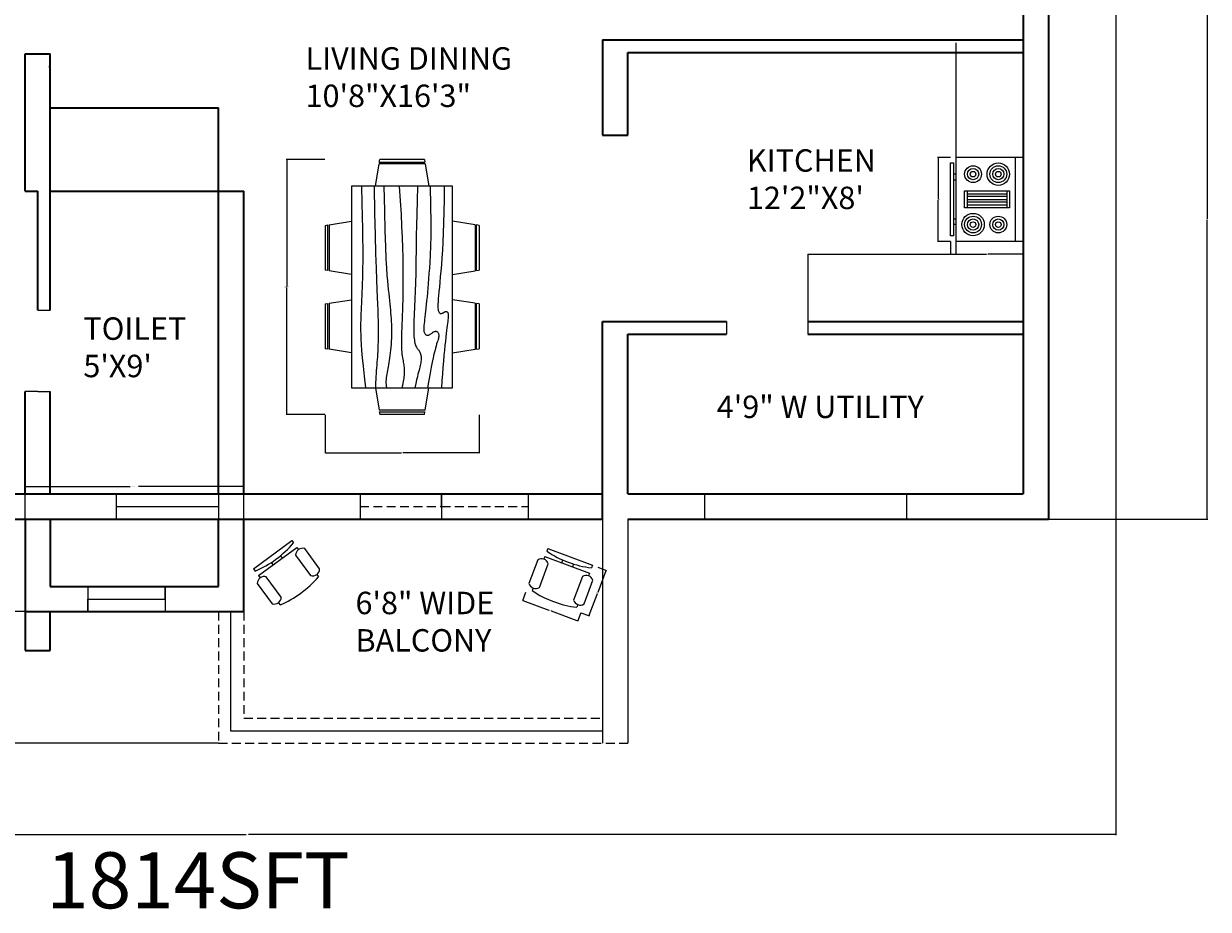
# Model space of a CAD drawing. Units: inches. Extents: x 514 to 1200, y -110 to 470.
# Tile 2 of 3: x 777 to 1200, y -110 to 206. Entities that reach past the tile are written whole.
import ezdxf

# ---------------------------------------------------------------- set-up
doc = ezdxf.new("R2010")
doc.units = ezdxf.units.IN
doc.linetypes.add('HIDDEN2', pattern=[4.7625, 3.175, -1.5875])
for name, color, linetype, lineweight in [('A-ANNO-DIMS', 2, 'Continuous', 18), ('A-ANNO-TEXT', 7, 'Continuous', 25), ('A-AREA-IDEN', 7, 'Continuous', 18), ('A-DOOR', 3, 'Continuous', 25), ('A-EQPM', 9, 'Continuous', 18), ('A-FLOR-FIXT', 9, 'Continuous', 18), ('A-FLOR-HIDN', 8, 'HIDDEN2', 18), ('A-FLOR-RAIL', 7, 'Continuous', 25), ('A-FURN', 8, 'Continuous', 18), ('A-GLAZ', 4, 'Continuous', 18), ('A-GLAZ-HIDN', 4, 'HIDDEN2', 18), ('A-WALL', 7, 'Continuous', 35)]:
    doc.layers.add(name, color=color, linetype=linetype, lineweight=lineweight)
doc.dimstyles.get("Standard").update_dxf_attribs({"dimtxt": 0.18, "dimasz": 0.18, "dimexe": 0.18, "dimexo": 0.0625, "dimgap": 0.09, "dimtad": 0, "dimtih": 1, "dimtoh": 1, "dimdec": 4, "dimzin": 0, "dimdsep": 46, "dimtxsty": 'Standard', "dimcen": 0.09, "dimadec": 0, "dimazin": 0, "dimtfac": 1, "dimtdec": 4, "dimtofl": 0, "dimtmove": 0, "dimatfit": 3, "dimfxl": 1, "dimtolj": 1, "dimtzin": 0, "dimarcsym": 0})

# ---------------------------------------------------------------- blocks, each defined once
blk = doc.blocks.new('Chair - Desk')
for p, q in [((-8.5, 0), (-8.5, -1)), ((-8.5, 0), (8.5, 0)), ((8.5, 0), (8.5, -1)), ((-8.5, -3), (-8.5, -4)), ((-8.5, -3), (8.5, -3)), ((-2, -3), (-2, -1.9355)), ((2, -1.9576), (2, -3)), ((8.5, -3), (8.5, -4)), ((-10.5, -5), (-10.5, -14)), ((-6.5, -14), (-6.5, -5)), ((6.5, -5), (6.5, -14)), ((10.5, -14), (10.5, -5)), ((-8.5, -15), (-8.5, -16)), ((8.5, -15), (8.5, -16))]:
    blk.add_line(p, q)
for centre, radius, start, end in [((-8.5, -6.5), 2.5, 36.8699, 143.1301), ((0, 34.625), 36.625, 256.5803, 283.4197), ((8.5, -6.5), 2.5, 36.8699, 143.1301), ((-8.5, -12.5), 2.5, 216.8699, 323.1301), ((0, 19.625), 36.625, 256.5803, 283.4197), ((8.5, -12.5), 2.5, 216.8699, 323.1301)]:
    blk.add_arc(centre, radius, start, end)
blk = doc.blocks.new('Dining Set - 36 x 72 in.')
for p, q in [((-22.2343, 26.00059), (-23.4847, 17.99762)), ((-22.2304, 26), (-5.7608, 26)), ((-22, 27.5), (-22.1562, 26.50042)), ((-5.8416, 26.5), (-22.1534, 26.5)), ((-22, 27.5), (-6, 27.5)), ((-5.8437, 26.49966), (-6, 27.5)), ((-4.5152, 17.99762), (-5.7655, 25.99926)), ((5.7657, 26.00059), (4.5153, 17.99762)), ((5.7696, 26), (22.2392, 26)), ((6, 27.5), (5.8438, 26.50042)), ((22.1584, 26.5), (5.8466, 26.5)), ((6, 27.5), (22, 27.5)), ((22.1563, 26.49966), (22, 27.5)), ((23.4848, 17.99762), (22.2345, 25.99926)), ((36, 18), (-36, 18)), ((-36, 18), (-36, -18)), ((36, -18), (36, 18)), ((-44.0006, 8.23428), (-35.9976, 9.48474)), ((44.0006, 8.23428), (35.9976, 9.48474)), ((-45.5, 8), (-44.5004, 8.15617)), ((-45.5, 8), (-45.5, -8)), ((-44.5, -8.15843), (-44.5, 8.15338)), ((-44, 8.23041), (-44, -8.23915)), ((44, 8.23041), (44, -8.23915)), ((44.5, -8.15843), (44.5, 8.15338)), ((45.5, 8), (44.5005, 8.15617)), ((45.5, 8), (45.5, -8)), ((-44.4997, -8.15631), (-45.5, -8)), ((-35.9976, -9.48476), (-43.9993, -8.2345)), ((35.9976, -9.48476), (43.9993, -8.2345)), ((44.4997, -8.15631), (45.5, -8)), ((-36, -18), (36, -18)), ((-22.2343, -26.0006), (-23.4847, -17.99762)), ((-4.5152, -17.99762), (-5.7655, -25.99928)), ((5.7657, -26.0006), (4.5153, -17.99762)), ((23.4848, -17.99762), (22.2345, -25.99928)), ((-22.2304, -26), (-5.7608, -26)), ((-22, -27.5), (-22.1562, -26.50044)), ((-5.8416, -26.5), (-22.1534, -26.5)), ((-22, -27.5), (-6, -27.5)), ((-5.8437, -26.49967), (-6, -27.5)), ((5.7696, -26), (22.2392, -26)), ((6, -27.5), (5.8438, -26.50044)), ((22.1584, -26.5), (5.8466, -26.5)), ((6, -27.5), (22, -27.5)), ((22.1563, -26.49967), (22, -27.5))]:
    blk.add_line(p, q)
for points in [[(-36, 15), (-31.1772, 14.97754), (-26.8079, 14.91406), (-22.8538, 14.81543), (-19.276, 14.6875), (-16.0362, 14.53613), (-13.0957, 14.36718), (-10.4159, 14.18652), (-7.9583, 14), (-5.6904, 13.81315), (-3.6035, 13.63021), (-1.6954, 13.45508), (0.0365, 13.29166), (1.5945, 13.14388), (2.9811, 13.01562), (4.1988, 12.9108), (5.25, 12.83333), (6.1393, 12.78613), (6.8802, 12.76823), (7.4883, 12.77767), (7.9792, 12.8125), (8.3685, 12.87077), (8.6719, 12.95052), (8.9049, 13.0498), (9.0833, 13.16666), (9.2205, 13.29899), (9.3216, 13.44401), (9.3895, 13.59879), (9.4271, 13.76041), (9.4373, 13.92594), (9.4232, 14.09245), (9.3875, 14.257), (9.3333, 14.41666), (9.2638, 14.56917), (9.1836, 14.71484), (9.0975, 14.85465), (9.0104, 14.98958), (8.9272, 15.1206), (8.8529, 15.2487), (8.7922, 15.37483), (8.75, 15.5), (8.7305, 15.62467), (8.7344, 15.74739), (8.7617, 15.86621), (8.8125, 15.97916), (8.8867, 16.08431), (8.9844, 16.17968), (9.1055, 16.26334), (9.25, 16.33333), (9.4189, 16.38802), (9.6172, 16.42708), (9.8506, 16.45052), (10.125, 16.45833), (10.4463, 16.45052), (10.8203, 16.42708), (11.2529, 16.38802), (11.75, 16.33333), (12.3184, 16.26318), (12.9694, 16.17838), (13.7151, 16.07991), (14.5677, 15.96875), (15.5395, 15.84586), (16.6426, 15.71224), (17.8893, 15.56884), (19.2917, 15.41666), (20.859, 15.25667), (22.5879, 15.08984), (24.4721, 14.91715), (26.5052, 14.73958), (28.6809, 14.5581), (30.9929, 14.3737), (33.4347, 14.18733), (36, 14)], [(-36, 10), (-28.9766, 10.14274), (-23.1725, 10.20442), (-18.4241, 10.19775), (-14.5677, 10.13541), (-11.4399, 10.03011), (-8.877, 9.89453), (-6.7154, 9.74137), (-4.7917, 9.58333), (-2.9698, 9.43082), (-1.2246, 9.28515), (0.4415, 9.14534), (2.026, 9.01041), (3.5266, 8.87939), (4.9408, 8.7513), (6.266, 8.62516), (7.5, 8.5), (8.6411, 8.37549), (9.6914, 8.2539), (10.6538, 8.13818), (11.5312, 8.03125), (12.3267, 7.93603), (13.043, 7.85547), (13.6831, 7.79248), (14.25, 7.75), (14.7471, 7.7303), (15.1797, 7.73307), (15.5537, 7.75732), (15.875, 7.80208), (16.1494, 7.86637), (16.3828, 7.94922), (16.5811, 8.04964), (16.75, 8.16666), (16.8944, 8.29915), (17.0143, 8.44531), (17.1089, 8.60319), (17.1771, 8.77083), (17.218, 8.94629), (17.2305, 9.1276), (17.2137, 9.31282), (17.1667, 9.5), (17.0895, 9.6875), (16.987, 9.875), (16.8649, 10.0625), (16.7292, 10.25), (16.5856, 10.4375), (16.4401, 10.625), (16.2985, 10.8125), (16.1667, 11), (16.05, 11.18733), (15.9518, 11.3737), (15.8752, 11.5581), (15.8229, 11.73958), (15.798, 11.91715), (15.8034, 12.08984), (15.842, 12.25667), (15.9167, 12.41666), (16.0295, 12.56836), (16.1784, 12.70833), (16.3605, 12.83268), (16.5729, 12.9375), (16.8127, 13.01888), (17.0768, 13.07291), (17.3625, 13.0957), (17.6667, 13.08333), (17.9894, 13.03312), (18.3418, 12.94726), (18.7382, 12.82918), (19.1927, 12.68229), (19.7195, 12.51001), (20.3327, 12.31575), (21.0465, 12.10294), (21.875, 11.875), (22.8357, 11.63354), (23.959, 11.37304), (25.2786, 11.08618), (26.8282, 10.76562), (28.6414, 10.40405), (30.752, 9.99414), (33.1936, 9.52856), (36, 9)], [(-36, 5.5), (-30.7157, 5.3348), (-26.069, 5.20963), (-21.9946, 5.11767), (-18.4271, 5.05208), (-15.3009, 5.00602), (-12.5508, 4.97265), (-10.1112, 4.94515), (-7.9167, 4.91666), (-5.909, 4.88167), (-4.0586, 4.83984), (-2.3429, 4.79215), (-0.7396, 4.73958), (0.7739, 4.6831), (2.22, 4.6237), (3.6213, 4.56233), (5, 4.5), (6.373, 4.43782), (7.7344, 4.3776), (9.0723, 4.32129), (10.375, 4.27083), (11.6309, 4.22819), (12.8281, 4.19531), (13.9551, 4.17415), (15, 4.16666), (15.954, 4.17448), (16.819, 4.19791), (17.6001, 4.23698), (18.3021, 4.29166), (18.9299, 4.36198), (19.4883, 4.44791), (19.9823, 4.54948), (20.4167, 4.66666), (20.7969, 4.79899), (21.1302, 4.94401), (21.4245, 5.09879), (21.6875, 5.26041), (21.9271, 5.42594), (22.1511, 5.59245), (22.3672, 5.757), (22.5834, 5.91666), (22.8065, 6.06868), (23.0404, 6.21093), (23.2879, 6.34147), (23.5521, 6.45833), (23.8358, 6.55957), (24.142, 6.64323), (24.4735, 6.70735), (24.8334, 6.75), (25.2235, 6.76969), (25.642, 6.76692), (26.0858, 6.74267), (26.5521, 6.69791), (27.0379, 6.63362), (27.5404, 6.55078), (28.0565, 6.45036), (28.5834, 6.33333), (29.1242, 6.19987), (29.7071, 6.04687), (30.3661, 5.87044), (31.1354, 5.66666), (32.0493, 5.43164), (33.142, 5.16146), (34.4475, 4.85221), (36, 4.5)], [(-36, -1), (-30.7915, -0.6591), (-26.0195, -0.38216), (-21.6519, -0.16284), (-17.6563, 0.00521), (-14.0005, 0.12833), (-10.6523, 0.21289), (-7.5796, 0.26522), (-4.75, 0.29166), (-2.134, 0.29793), (0.2878, 0.28711), (2.5317, 0.26163), (4.6146, 0.22396), (6.5529, 0.17651), (8.3633, 0.12174), (10.0623, 0.06209), (11.6667, 0), (13.1899, -0.06201), (14.6341, -0.1211), (15.9982, -0.17432), (17.2813, -0.21875), (18.4823, -0.25147), (19.6003, -0.26953), (20.6343, -0.27002), (21.5834, -0.25), (22.4481, -0.20768), (23.2357, -0.14584), (23.9549, -0.06836), (24.6146, 0.02083), (25.2235, 0.11784), (25.7904, 0.21875), (26.3241, 0.31966), (26.8334, 0.41666), (27.3265, 0.50618), (27.8099, 0.58593), (28.2894, 0.65397), (28.7709, 0.70833), (29.2601, 0.74707), (29.763, 0.76823), (30.2855, 0.76985), (30.8334, 0.75), (31.4088, 0.70784), (31.9994, 0.64713), (32.589, 0.57275), (33.1615, 0.48958), (33.7008, 0.4025), (34.1908, 0.3164), (34.6153, 0.23616), (34.9584, 0.16666), (35.2099, 0.11165), (35.3848, 0.07031), (35.504, 0.04069), (35.5886, 0.02083), (35.6594, 0.00879), (35.7377, 0.0026), (35.8442, 0.00032), (36, 0)], [(-36, -6.5), (-27.1843, -6.31267), (-20.084, -6.1263), (-14.469, -5.9419), (-10.1094, -5.76042), (-6.7752, -5.58285), (-4.2363, -5.41016), (-2.2629, -5.24333), (-0.625, -5.08334), (0.8708, -4.93099), (2.2715, -4.78646), (3.5872, -4.64974), (4.8281, -4.52084), (6.0046, -4.39974), (7.127, -4.28646), (8.2053, -4.18099), (9.25, -4.08334), (10.2705, -3.99382), (11.2734, -3.91407), (12.2647, -3.84603), (13.25, -3.79167), (14.2354, -3.75293), (15.2266, -3.73177), (16.2295, -3.73015), (17.25, -3.75), (18.2912, -3.79248), (19.3451, -3.85547), (20.4009, -3.93604), (21.4479, -4.03125), (22.4754, -4.13819), (23.4727, -4.25391), (24.4289, -4.37549), (25.3334, -4.5), (26.1785, -4.62492), (26.9694, -4.74935), (27.7145, -4.87281), (28.4219, -4.99479), (29.1, -5.11483), (29.7572, -5.23242), (30.4016, -5.34709), (31.0417, -5.45834), (31.6837, -5.56437), (32.3262, -5.65821), (32.9658, -5.73153), (33.599, -5.77604), (34.2224, -5.78345), (34.8327, -5.74545), (35.4264, -5.65373), (36, -5.5)], [(-36, -10), (-26.4022, -9.81299), (-18.4675, -9.62891), (-11.9839, -9.45069), (-6.7396, -9.28125), (-2.5226, -9.12354), (0.8789, -8.98047), (3.6769, -8.85498), (6.0833, -8.75), (8.2767, -8.66765), (10.3021, -8.60677), (12.1712, -8.56543), (13.8958, -8.54167), (15.4876, -8.53353), (16.9583, -8.53907), (18.3197, -8.55632), (19.5834, -8.58334), (20.7616, -8.61841), (21.8685, -8.66081), (22.9188, -8.71004), (23.9271, -8.76563), (24.9081, -8.82707), (25.8763, -8.89388), (26.8465, -8.96558), (27.8334, -9.04167), (28.8474, -9.12118), (29.8828, -9.20117), (30.93, -9.27824), (31.9792, -9.34896), (33.0205, -9.40991), (34.0443, -9.45768), (35.0407, -9.48885), (36, -9.5)], [(-36, -14.5), (-30.0881, -14.33513), (-25.0332, -14.21224), (-20.7312, -14.12647), (-17.0781, -14.07292), (-13.97, -14.04671), (-11.3027, -14.04297), (-8.9724, -14.05681), (-6.875, -14.08334), (-4.9224, -14.11833), (-3.0905, -14.16016), (-1.3709, -14.20785), (0.2448, -14.26042), (1.7647, -14.3169), (3.1973, -14.3763), (4.5507, -14.43767), (5.8333, -14.5), (7.0554, -14.5621), (8.235, -14.62175), (9.3922, -14.67652), (10.5469, -14.72396), (11.7192, -14.76164), (12.929, -14.78711), (14.1965, -14.79794), (15.5417, -14.79167), (16.9933, -14.76424), (18.6152, -14.70508), (20.4804, -14.60197), (22.6615, -14.44271), (25.2312, -14.21509), (28.2624, -13.9069), (31.8277, -13.50594), (36, -13)]]:
    blk.add_lwpolyline(points)
blk = doc.blocks.new('Range-Oven - 30 in top')
for p, q in [((0, -3), (30, -3)), ((12, -6), (18, -6)), ((13, -20), (13, -6)), ((14, -6), (14, -20)), ((15, -20), (15, -6)), ((16, -6), (16, -20)), ((17, -20), (17, -6)), ((18, -20), (12, -20)), ((6, -24), (6, -25)), ((8, -25), (8, -24)), ((22, -25), (22, -24)), ((24, -24), (24, -25))]:
    blk.add_line(p, q)
for points in [[(0, -24), (0, 0), (30, 0), (30, -24)], [(12, -21), (12, -5), (18, -5), (18, -21)], [(2, -26), (2, -25), (28, -25), (28, -26)]]:
    blk.add_lwpolyline(points, close=True)
for centre, radius in [((6, -9), 4), ((6, -9), 3), ((6, -9), 2), ((6, -9), 1), ((24, -9), 3), ((24, -9), 2), ((24, -9), 1), ((6, -18), 3), ((6, -18), 2), ((24, -18), 4), ((24, -18), 3), ((24, -18), 2), ((6, -18), 1), ((24, -18), 1)]:
    blk.add_circle(centre, radius)
blk = doc.blocks.new('WALL-BAY-60x24')
for p, q in [((0, 33), (0, 0)), ((9, 33), (9, 9)), ((69, 9), (69, 33)), ((78, 0), (78, 33)), ((9, 9), (69, 9)), ((0, 0), (78, 0))]:
    blk.add_line(p, q)
blk = doc.blocks.new('*D10')
at = {"layer": 'A-ANNO-DIMS', "color": 0, "lineweight": -2, "transparency": 16777216}
for p, q in [((956.39, 2.9), (955.25, -0.16)), ((955.48, -0.06), (964.67, -3.48)), ((974.82, -7.26), (965.64, -3.84)), ((976.07, -4.43), (974.93, -7.49))]:
    blk.add_line(p, q, dxfattribs=at)
at = {"layer": 'A-ANNO-DIMS', "color": 0, "transparency": 16777216}
for points in [[(955.49, -0.03), (955.47, -0.09), (955.31, 0)], [(974.83, -7.23), (974.81, -7.29), (974.99, -7.32)]]:
    blk.add_solid(points, dxfattribs=at)
at = {"layer": 'Defpoints', "color": 0, "transparency": 16777216}
for p in [(956.41, 2.96), (974.99, -7.32), (976.09, -4.37)]:
    blk.add_point(p, dxfattribs=at)
at = {"layer": 'A-ANNO-DIMS', "color": 0, "transparency": 16777216, "insert": (965.15, -3.66), "char_height": 0.18, "attachment_point": 5}
blk.add_mtext('\\A1;CHAIR 21 TYP.', dxfattribs=at)
blk = doc.blocks.new('*D11')
at = {"layer": 'A-ANNO-DIMS', "color": 0, "lineweight": -2, "transparency": 16777216}
for p, q in [((985.03, 10.61), (982.13, 2.83)), ((982.2, 11.85), (985.26, 10.71)), ((979.11, -5.3), (982, 2.47)), ((976.15, -4.39), (979.21, -5.53))]:
    blk.add_line(p, q, dxfattribs=at)
at = {"layer": 'A-ANNO-DIMS', "color": 0, "transparency": 16777216}
for points in [[(985, 10.62), (985.06, 10.6), (985.09, 10.78)], [(979.08, -5.29), (979.13, -5.31), (979.04, -5.47)]]:
    blk.add_solid(points, dxfattribs=at)
at = {"layer": 'Defpoints', "color": 0, "transparency": 16777216}
for p in [(982.14, 11.88), (985.09, 10.78), (976.09, -4.37)]:
    blk.add_point(p, dxfattribs=at)
at = {"layer": 'A-ANNO-DIMS', "color": 0, "transparency": 16777216, "insert": (982.07, 2.65), "char_height": 0.18, "attachment_point": 5}
blk.add_mtext('\\A1;17 TYP.', dxfattribs=at)
blk = doc.blocks.new('*D16')
at = {"layer": 'A-ANNO-DIMS', "color": 0, "lineweight": -2, "transparency": 16777216}
for p, q in [((777.89, 29.08), (777.89, 40.9)), ((778.07, 40.72), (815.42, 40.72)), ((855.71, 40.72), (818.36, 40.72)), ((855.89, 29.08), (855.89, 40.9))]:
    blk.add_line(p, q, dxfattribs=at)
at = {"layer": 'A-ANNO-DIMS', "color": 0, "transparency": 16777216}
for points in [[(778.07, 40.75), (778.07, 40.69), (777.89, 40.72)], [(855.71, 40.75), (855.71, 40.69), (855.89, 40.72)]]:
    blk.add_solid(points, dxfattribs=at)
at = {"layer": 'Defpoints', "color": 0, "transparency": 16777216}
for p in [(855.89, 40.72), (777.89, 29.02), (855.89, 29.02)]:
    blk.add_point(p, dxfattribs=at)
at = {"layer": 'A-ANNO-DIMS', "color": 0, "transparency": 16777216, "insert": (816.89, 40.72), "char_height": 0.18, "attachment_point": 5}
blk.add_mtext('\\A1;WALL BAY 78 TYP.', dxfattribs=at)
blk = doc.blocks.new('*D17')
at = {"layer": 'A-ANNO-DIMS', "color": 0, "lineweight": -2, "transparency": 16777216}
for p, q in [((777.83, 29.02), (766.01, 29.02)), ((766.19, 28.84), (766.19, 12.7)), ((766.19, -3.8), (766.19, 12.34)), ((777.83, -3.98), (766.01, -3.98))]:
    blk.add_line(p, q, dxfattribs=at)
at = {"layer": 'A-ANNO-DIMS', "color": 0, "transparency": 16777216}
for points in [[(766.16, 28.84), (766.22, 28.84), (766.19, 29.02)], [(766.16, -3.8), (766.22, -3.8), (766.19, -3.98)]]:
    blk.add_solid(points, dxfattribs=at)
at = {"layer": 'Defpoints', "color": 0, "transparency": 16777216}
for p in [(766.19, 29.02), (777.89, 29.02), (777.89, -3.98)]:
    blk.add_point(p, dxfattribs=at)
at = {"layer": 'A-ANNO-DIMS', "color": 0, "transparency": 16777216, "insert": (766.19, 12.52), "char_height": 0.18, "attachment_point": 5}
blk.add_mtext('\\A1;33 TYP.', dxfattribs=at)
blk = doc.blocks.new('*D20')
at = {"layer": 'A-ANNO-DIMS', "color": 0, "lineweight": -2, "transparency": 16777216}
for p, q in [((884.8, 157.35), (871.03, 157.35)), ((871.21, 157.17), (871.21, 112.03)), ((871.21, 66.53), (871.21, 111.67)), ((884.8, 66.35), (871.03, 66.35))]:
    blk.add_line(p, q, dxfattribs=at)
at = {"layer": 'A-ANNO-DIMS', "color": 0, "transparency": 16777216}
for points in [[(871.18, 157.17), (871.24, 157.17), (871.21, 157.35)], [(871.18, 66.53), (871.24, 66.53), (871.21, 66.35)]]:
    blk.add_solid(points, dxfattribs=at)
at = {"layer": 'Defpoints', "color": 0, "transparency": 16777216}
for p in [(884.86, 157.35), (871.21, 66.35), (884.86, 66.35)]:
    blk.add_point(p, dxfattribs=at)
at = {"layer": 'A-ANNO-DIMS', "color": 0, "transparency": 16777216, "insert": (871.21, 111.85), "char_height": 0.18, "attachment_point": 5}
blk.add_mtext('\\A1;DINING SET 91', dxfattribs=at)
blk = doc.blocks.new('*D21')
at = {"layer": 'A-ANNO-DIMS', "color": 0, "lineweight": -2, "transparency": 16777216}
for p, q in [((884.86, 66.29), (884.86, 52.52)), ((939.86, 66.29), (939.86, 52.52)), ((885.04, 52.7), (912.12, 52.7)), ((939.68, 52.7), (912.6, 52.7))]:
    blk.add_line(p, q, dxfattribs=at)
at = {"layer": 'A-ANNO-DIMS', "color": 0, "transparency": 16777216}
for points in [[(885.04, 52.73), (885.04, 52.67), (884.86, 52.7)], [(939.68, 52.73), (939.68, 52.67), (939.86, 52.7)]]:
    blk.add_solid(points, dxfattribs=at)
at = {"layer": 'Defpoints', "color": 0, "transparency": 16777216}
for p in [(884.86, 66.35), (939.86, 66.35), (939.86, 52.7)]:
    blk.add_point(p, dxfattribs=at)
at = {"layer": 'A-ANNO-DIMS', "color": 0, "transparency": 16777216, "insert": (912.36, 52.7), "char_height": 0.18, "attachment_point": 5}
blk.add_mtext('\\A1;55', dxfattribs=at)
blk = doc.blocks.new('*D22')
at = {"layer": 'A-ANNO-DIMS', "color": 0, "lineweight": -2, "transparency": 16777216}
for p, q in [((1107.95, 158.13), (1103.33, 158.13)), ((1103.51, 157.95), (1103.51, 143.31)), ((1103.51, 128.31), (1103.51, 142.95)), ((1107.95, 128.13), (1103.33, 128.13))]:
    blk.add_line(p, q, dxfattribs=at)
at = {"layer": 'A-ANNO-DIMS', "color": 0, "transparency": 16777216}
for points in [[(1103.48, 157.95), (1103.54, 157.95), (1103.51, 158.13)], [(1103.48, 128.31), (1103.54, 128.31), (1103.51, 128.13)]]:
    blk.add_solid(points, dxfattribs=at)
at = {"layer": 'Defpoints', "color": 0, "transparency": 16777216}
for p in [(1108.01, 158.13), (1103.51, 128.13), (1108.01, 128.13)]:
    blk.add_point(p, dxfattribs=at)
at = {"layer": 'A-ANNO-DIMS', "color": 0, "transparency": 16777216, "insert": (1103.51, 143.13), "char_height": 0.18, "attachment_point": 5}
blk.add_mtext('\\A1;RANGE 30', dxfattribs=at)
blk = doc.blocks.new('*D23')
at = {"layer": 'A-ANNO-DIMS', "color": 0, "lineweight": -2, "transparency": 16777216}
for p, q in [((1108.01, 128.07), (1108.01, 123.45)), ((1134.01, 128.07), (1134.01, 123.45)), ((1108.19, 123.63), (1120.77, 123.63)), ((1133.83, 123.63), (1121.25, 123.63))]:
    blk.add_line(p, q, dxfattribs=at)
at = {"layer": 'A-ANNO-DIMS', "color": 0, "transparency": 16777216}
for points in [[(1108.19, 123.66), (1108.19, 123.6), (1108.01, 123.63)], [(1133.83, 123.66), (1133.83, 123.6), (1134.01, 123.63)]]:
    blk.add_solid(points, dxfattribs=at)
at = {"layer": 'Defpoints', "color": 0, "transparency": 16777216}
for p in [(1108.01, 128.13), (1134.01, 128.13), (1134.01, 123.63)]:
    blk.add_point(p, dxfattribs=at)
at = {"layer": 'A-ANNO-DIMS', "color": 0, "transparency": 16777216, "insert": (1121.01, 123.63), "char_height": 0.18, "attachment_point": 5}
blk.add_mtext('\\A1;26', dxfattribs=at)
blk = doc.blocks.new('*D35')
at = {"layer": 'A-ANNO-DIMS', "color": 0, "lineweight": -2, "transparency": 16777216}
for p, q in [((1142.953064, 243.070714), (1199.719295, 243.070714)), ((1199.539295, 242.890714), (1199.539295, 136.225705)), ((1199.539295, 29.200696), (1199.539295, 135.865705)), ((1142.953064, 29.020696), (1199.719295, 29.020696))]:
    blk.add_line(p, q, dxfattribs=at)
at = {"layer": 'A-ANNO-DIMS', "color": 0, "transparency": 16777216}
for points in [[(1199.509295, 242.890714), (1199.569295, 242.890714), (1199.539295, 243.070714)], [(1199.509295, 29.200696), (1199.569295, 29.200696), (1199.539295, 29.020696)]]:
    blk.add_solid(points, dxfattribs=at)
at = {"layer": 'Defpoints', "color": 0, "transparency": 16777216}
for p in [(1142.890564, 243.070714), (1142.890564, 29.020696), (1199.539295, 29.020696)]:
    blk.add_point(p, dxfattribs=at)
at = {"layer": 'A-ANNO-DIMS', "color": 0, "transparency": 16777216, "insert": (1199.539295, 136.045705), "char_height": 0.18, "attachment_point": 5}
blk.add_mtext('\\A1;214.05', dxfattribs=at)
blk = doc.blocks.new('*D36')
at = {"layer": 'A-ANNO-DIMS', "color": 0, "lineweight": -2, "transparency": 16777216}
for p, q in [((1166.99, 243.01), (1166.99, -83.71)), ((547.32, 185.96), (547.32, -83.71)), ((547.5, -83.53), (856.73, -83.53)), ((1166.81, -83.53), (857.57, -83.53))]:
    blk.add_line(p, q, dxfattribs=at)
at = {"layer": 'A-ANNO-DIMS', "color": 0, "transparency": 16777216}
for points in [[(547.5, -83.5), (547.5, -83.56), (547.32, -83.53)], [(1166.81, -83.5), (1166.81, -83.56), (1166.99, -83.53)]]:
    blk.add_solid(points, dxfattribs=at)
at = {"layer": 'Defpoints', "color": 0, "transparency": 16777216}
for p in [(1166.99, 243.07), (547.32, 186.02), (1166.99, -83.53)]:
    blk.add_point(p, dxfattribs=at)
at = {"layer": 'A-ANNO-DIMS', "color": 0, "transparency": 16777216, "insert": (857.15, -83.53), "char_height": 0.18, "attachment_point": 5}
blk.add_mtext('\\A1;619.7', dxfattribs=at)
blk = doc.blocks.new('*D37')
at = {"layer": 'A-ANNO-DIMS', "color": 0, "lineweight": -2, "transparency": 16777216}
for p, q in [((719.82324, 437.520696), (514.588716, 437.520696)), ((514.768716, 437.340696), (514.768716, 193.450696)), ((514.768716, -50.799304), (514.768716, 193.090696)), ((846.828064, -50.979304), (514.588716, -50.979304))]:
    blk.add_line(p, q, dxfattribs=at)
at = {"layer": 'A-ANNO-DIMS', "color": 0, "transparency": 16777216}
for points in [[(514.738716, 437.340696), (514.798716, 437.340696), (514.768716, 437.520696)], [(514.738716, -50.799304), (514.798716, -50.799304), (514.768716, -50.979304)]]:
    blk.add_solid(points, dxfattribs=at)
at = {"layer": 'Defpoints', "color": 0, "transparency": 16777216}
for p in [(514.768716, 437.520696), (719.88574, 437.520696), (846.890564, -50.979304)]:
    blk.add_point(p, dxfattribs=at)
at = {"layer": 'A-ANNO-DIMS', "color": 0, "transparency": 16777216, "insert": (514.768716, 193.270696), "char_height": 0.18, "attachment_point": 5}
blk.add_mtext('\\A1;488.5', dxfattribs=at)

msp = doc.modelspace()

# ---------------------------------------------------------------- linework, layer by layer
at = {"layer": 'A-DOOR'}
for p, q in [((782.3906, 103.5553), (786.8906, 103.5553)), ((1028.1021, 99.5207), (1028.1021, 95.0207)), ((1057.1021, 99.5207), (1057.1021, 95.0207)), ((782.3906, 74.5553), (777.8906, 74.5553)), ((782.3906, 74.5553), (786.8906, 74.5553))]:
    msp.add_line(p, q, dxfattribs=at)
at = {"layer": 'A-FLOR-FIXT'}
for p, q in [((1109.8906, 199.0207), (1109.8906, 123.5207)), ((1057.1021, 123.5207), (1109.8906, 123.5207)), ((1057.1021, 123.5207), (1057.1021, 99.5207))]:
    msp.add_line(p, q, dxfattribs=at)
at = {"layer": 'A-FLOR-HIDN'}
for p, q in [((846.8906, -3.9793), (846.8906, -50.9793)), ((855.8906, -3.9793), (855.8906, -41.9793)), ((855.8906, -41.9793), (983.8906, -41.9793)), ((846.8906, -50.9793), (992.8906, -50.9793))]:
    msp.add_line(p, q, dxfattribs=at)
at = {"layer": 'A-FLOR-RAIL'}
for p, q in [((983.8906, 29.0207), (983.8906, -41.9793)), ((992.8906, 29.0207), (992.8906, -50.9793)), ((851.1942, -3.9793), (851.1942, -46.5438)), ((983.8906, -41.9793), (983.8906, -50.9793)), ((851.1942, -46.5438), (983.8906, -46.5438))]:
    msp.add_line(p, q, dxfattribs=at)
at = {"layer": 'A-GLAZ'}
for p, q in [((810.3821, 38.0207), (810.3821, 29.0207)), ((846.8906, 38.0207), (846.8906, 29.0207)), ((897.3578, 38.0207), (897.3578, 29.0207)), ((926.4279, 33.5207), (926.4279, 38.0207)), ((926.4279, 38.0207), (926.4279, 29.0207)), ((957.3578, 38.0207), (957.3578, 29.0207)), ((1020.2649, 38.0207), (1020.2649, 29.0207)), ((1092.2649, 38.0207), (1092.2649, 29.0207)), ((810.3821, 33.5207), (846.8906, 33.5207)), ((800.2296, 5.0207), (800.2296, -3.9793)), ((827.8585, 0.5207), (827.8585, 5.0207)), ((827.8585, 5.0207), (827.8585, -3.9793)), ((800.2296, -3.9793), (800.2296, 0.5207)), ((800.2296, 0.5207), (827.8585, 0.5207))]:
    msp.add_line(p, q, dxfattribs=at)
at = {"layer": 'A-GLAZ-HIDN'}
for p, q in [((897.3578, 33.5207), (926.4279, 33.5207)), ((926.4279, 33.5207), (957.3578, 33.5207))]:
    msp.add_line(p, q, dxfattribs=at)
at = {"layer": 'A-WALL'}
for p, q in [((1133.8906, 255.0207), (1133.8906, 199.0207)), ((1142.8906, 255.0207), (1142.8906, 199.0207)), ((983.8906, 200.0207), (1133.8906, 200.0207)), ((983.8906, 200.0207), (983.8906, 192.217)), ((1133.8906, 199.0207), (1133.8906, 38.0207)), ((1142.8906, 199.0207), (1142.8906, 38.0207)), ((777.8906, 146.0207), (777.8906, 195.0207)), ((777.8906, 195.0207), (786.3906, 195.0207)), ((786.3906, 195.0207), (786.8906, 195.0207)), ((786.8906, 103.5553), (786.8906, 195.0207)), ((983.8906, 195.5207), (983.8906, 166.0499)), ((992.8906, 195.5207), (1133.8906, 195.5207)), ((992.8906, 166.0499), (992.8906, 195.5207)), ((1057.1021, 195.5207), (1133.8906, 195.5207)), ((786.3906, 190.5207), (786.8906, 190.5207)), ((786.8906, 175.7456), (846.8906, 175.7456)), ((846.8906, 38.0207), (846.8906, 175.7456)), ((983.8906, 166.0499), (992.8906, 166.0499)), ((777.8906, 146.0207), (782.3906, 146.0207)), ((782.3906, 103.5553), (782.3906, 146.0207)), ((786.8906, 146.0207), (855.8906, 146.0207)), ((855.8906, 38.0207), (855.8906, 146.0207)), ((983.8906, 95.0207), (983.8906, 99.5207)), ((983.8906, 99.5207), (1028.1021, 99.5207)), ((1057.1021, 99.5207), (1133.8906, 99.5207)), ((983.8906, 29.0207), (983.8906, 95.0207)), ((992.8906, 38.0207), (992.8906, 95.0207)), ((992.8906, 95.0207), (1028.1021, 95.0207)), ((1057.1021, 95.0207), (1133.8906, 95.0207)), ((777.8906, 38.0207), (777.8906, 74.5553)), ((786.8906, 38.0207), (786.8906, 74.5553)), ((609.8906, 38.0207), (983.8906, 38.0207)), ((992.8906, 38.0207), (1133.8906, 38.0207)), ((1142.8906, 38.0207), (1142.8906, 29.0207)), ((600.8906, 29.0207), (983.8906, 29.0207)), ((992.8906, 29.0207), (1142.8906, 29.0207)), ((777.8906, -3.9793), (777.8906, -17.8235)), ((786.8906, -17.8235), (786.8906, -3.9793)), ((777.8906, -17.8235), (786.8906, -17.8235))]:
    msp.add_line(p, q, dxfattribs=at)

# ---------------------------------------------------------------- block references
at = {"layer": 'A-EQPM', "rotation": 270}
msp.add_blockref('Range-Oven - 30 in top', (1134.0098, 158.1334), dxfattribs=at)
at = {"layer": 'A-FURN'}
for name, p, rotation in [('Dining Set - 36 x 72 in.', (912.3633, 111.8535), 270), ('Chair - Desk', (866.1906, 16.3122), 36.38435206520505), ('Chair - Desk', (972.2974, 15.5382), 339.5846014925849)]:
    msp.add_blockref(name, p, dxfattribs=dict(at, rotation=rotation))
at = {"layer": 'A-WALL'}
msp.add_blockref('WALL-BAY-60x24', (777.8906, -3.9793), dxfattribs=at)

# ---------------------------------------------------------------- texts
at = {"layer": 'A-ANNO-TEXT', "insert": (785.4568, -89.8564), "char_height": 20, "attachment_point": 1}
msp.add_mtext_dynamic_manual_height_columns('{\\fTimes New Roman|b0|i0|c0|p18;1814SFT}', width=92.773282, gutter_width=12.5, heights=[0], dxfattribs=at)
at = {"layer": 'A-AREA-IDEN', "char_height": 8, "attachment_point": 1}
for s, insert in [('{\\fTimes New Roman|b0|i0|c0|p18;LIVING DINING\\P10\'8"X16\'3"}', (877.9248, 197.4241)), ('{\\fTimes New Roman|b0|i0|c0|p18;KITCHEN\\P12\'2"X8\'}', (1035.3455, 161.0022)), ("{\\fTimes New Roman|b0|i0|c0|p18;TOILET\\P5'X9'}", (798.6756, 101.0092)), ('{\\fTimes New Roman|b0|i0|c0|p18;4\'9" W UTILITY}', (1024.5924, 73.1003)), ('{\\fTimes New Roman|b0|i0|c0|p18;6\'8" WIDE BALCONY}', (895.7364, 3.1038))]:
    msp.add_mtext_dynamic_manual_height_columns(s, width=92.773282, gutter_width=12.5, heights=[0], dxfattribs=dict(at, insert=insert))

# ---------------------------------------------------------------- dimensions: what is measured, and where the dimension line sits
at = {"layer": 'A-ANNO-DIMS'}
for base, p1, p2, override, picture, middle in [((514.7687, 437.5207), (846.8906, -50.9793), (719.8857, 437.5207), {"dimdec": 1, "dimlfac": 1, "dimrnd": 0, "dimzin": 0, "dimdsep": 46, "dimlunit": 2}, '*D37', (514.7687, 193.2707)), ((1199.5393, 29.0207), (1142.8906, 243.0707), (1142.8906, 29.0207), {"dimdec": 2, "dimlfac": 1, "dimrnd": 0, "dimzin": 0, "dimdsep": 46, "dimlunit": 2}, '*D35', (1199.5393, 136.0457))]:
    dim = msp.add_linear_dim(base=base, p1=p1, p2=p2, angle=90, dimstyle='Standard', override=override, dxfattribs=at)
    dim.commit()
    dim.dimension.update_dxf_attribs({"geometry": picture, "text_midpoint": middle})
for base, p1, p2, override, picture, middle in [((1166.9893, -83.5293), (547.3187, 186.0207), (1166.9893, 243.0707), {"dimdec": 1, "dimlfac": 1, "dimrnd": 0, "dimzin": 0, "dimdsep": 46, "dimlunit": 2}, '*D36', (857.154, -83.5293)), ((1134.0098, 123.6334), (1108.0098, 128.1334), (1134.0098, 128.1334), {"dimdec": 0, "dimlfac": 1, "dimrnd": 0, "dimzin": 0, "dimdsep": 46, "dimlunit": 2}, '*D23', (1121.0098, 123.6334)), ((939.8633, 52.7035), (884.8633, 66.3535), (939.8633, 66.3535), {"dimdec": 0, "dimlfac": 1, "dimrnd": 0, "dimzin": 0, "dimdsep": 46, "dimlunit": 2}, '*D21', (912.3633, 52.7035))]:
    dim = msp.add_linear_dim(base=base, p1=p1, p2=p2, dimstyle='Standard', override=override, dxfattribs=at)
    dim.commit()
    dim.dimension.update_dxf_attribs({"geometry": picture, "text_midpoint": middle})
for base, p1, p2, angle, text, picture, middle in [((871.2133, 66.3535), (884.8633, 157.3535), (884.8633, 66.3535), 270, 'DINING SET <>', '*D20', (871.2133, 111.8535)), ((1103.5098, 128.1334), (1108.0098, 158.1334), (1108.0098, 128.1334), 270, 'RANGE <>', '*D22', (1103.5098, 143.1334)), ((766.1906, 29.0207), (777.8906, -3.9793), (777.8906, 29.0207), 90, '<> TYP.', '*D17', (766.1906, 12.5207)), ((985.09, 10.7768), (976.0916, -4.369), (982.1379, 11.8756), 69.584601, '<> TYP.', '*D11', (982.0669, 2.6545)), ((974.9928, -7.3212), (956.4107, 2.9563), (976.0916, -4.369), 339.584601, 'CHAIR <> TYP.', '*D10', (965.1523, -3.6585))]:
    dim = msp.add_linear_dim(base=base, p1=p1, p2=p2, angle=angle, text=text, dimstyle='Standard', override={"dimdec": 0, "dimlfac": 1, "dimrnd": 0, "dimzin": 0, "dimdsep": 46, "dimlunit": 2}, dxfattribs=at)
    dim.commit()
    dim.dimension.update_dxf_attribs({"geometry": picture, "text_midpoint": middle})
dim = msp.add_linear_dim(base=(855.8906, 40.7207), p1=(777.8906, 29.0207), p2=(855.8906, 29.0207), text='WALL BAY <> TYP.', dimstyle='Standard', override={"dimdec": 0, "dimlfac": 1, "dimrnd": 0, "dimzin": 0, "dimdsep": 46, "dimlunit": 2}, dxfattribs=at)
dim.commit()
dim.dimension.update_dxf_attribs({"geometry": '*D16', "text_midpoint": (816.8906, 40.7207)})

doc.saveas('drawing.dxf')
